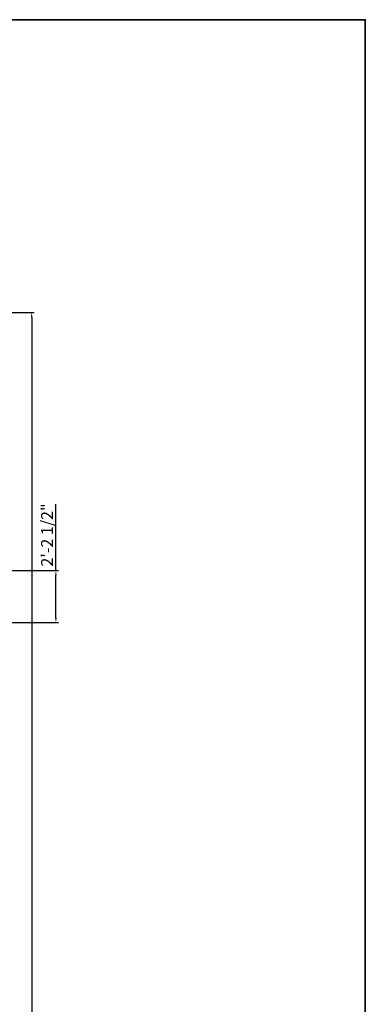
# Model space of a CAD drawing. Units: inches. Extents: x 2123 to 2977, y 1464 to 2698.
# Tile 10 of 10: x 2801 to 2977, y 2196 to 2698. Entities that reach past the tile are written whole.
import ezdxf

# ---------------------------------------------------------------- set-up
doc = ezdxf.new("R2010")
doc.units = ezdxf.units.IN
doc.layers.add('A-ANNO-DIMS', color=2, linetype='Continuous', lineweight=18)
doc.layers.add('A-ANNO-TTLB', color=7, linetype='Continuous', lineweight=35)
doc.styles.get("Standard").update_dxf_attribs({"font": 'arial.ttf'})
doc.dimstyles.new('ISO-25', dxfattribs={"dimtxt": 6, "dimasz": 2.5, "dimexe": 1.25, "dimexo": 0.625, "dimtad": 1, "dimdec": 0, "dimlunit": 3, "dimtxsty": 'Standard', "dimcen": 2.5, "dimadec": 0, "dimazin": 0, "dimtfac": 1, "dimtdec": 0, "dimtmove": 0, "dimatfit": 3, "dimfxl": 1, "dimarcsym": 0})

# ---------------------------------------------------------------- blocks, each defined once
blk = doc.blocks.new('*D9')
at = {"layer": 'A-ANNO-DIMS', "color": 0, "lineweight": -2, "transparency": 16777216}
for p, q in [((2767.56, 2548.37), (2808.58, 2548.37)), ((2807.33, 2545.87), (2807.33, 1686.46)), ((2767.56, 1683.96), (2808.58, 1683.96))]:
    blk.add_line(p, q, dxfattribs=at)
at = {"layer": 'A-ANNO-DIMS', "color": 0, "transparency": 16777216}
for points in [[(2806.91, 2545.87), (2807.74, 2545.87), (2807.33, 2548.37)], [(2806.91, 1686.46), (2807.74, 1686.46), (2807.33, 1683.96)]]:
    blk.add_solid(points, dxfattribs=at)
at = {"layer": 'Defpoints', "color": 0, "transparency": 16777216}
for p in [(2766.94, 2548.37), (2766.94, 1683.96), (2807.33, 1683.96)]:
    blk.add_point(p, dxfattribs=at)
at = {"layer": 'A-ANNO-DIMS', "color": 0, "transparency": 16777216, "insert": (2803.69, 2116.16), "char_height": 6, "attachment_point": 5, "rotation": 90}
blk.add_mtext("72'", dxfattribs=at)
blk = doc.blocks.new('*D59')
at = {"layer": 'A-ANNO-DIMS', "color": 0, "lineweight": -2, "transparency": 16777216}
for p, q in [((2819.64, 2416.87), (2819.64, 2450.65)), ((2376.14, 2416.87), (2820.89, 2416.87)), ((2819.64, 2392.84), (2819.64, 2414.37)), ((2344.56, 2390.34), (2820.89, 2390.34))]:
    blk.add_line(p, q, dxfattribs=at)
at = {"layer": 'A-ANNO-DIMS', "color": 0, "transparency": 16777216}
for points in [[(2819.22, 2414.37), (2820.05, 2414.37), (2819.64, 2416.87)], [(2819.22, 2392.84), (2820.05, 2392.84), (2819.64, 2390.34)]]:
    blk.add_solid(points, dxfattribs=at)
at = {"layer": 'Defpoints', "color": 0, "transparency": 16777216}
for p in [(2375.52, 2416.87), (2819.64, 2416.87), (2343.94, 2390.34)]:
    blk.add_point(p, dxfattribs=at)
at = {"layer": 'A-ANNO-DIMS', "color": 0, "transparency": 16777216, "insert": (2815.91, 2435.01), "char_height": 6, "attachment_point": 5, "rotation": 90}
blk.add_mtext('2\'-2 1/2"', dxfattribs=at)

msp = doc.modelspace()

# ---------------------------------------------------------------- linework, layer by layer
at = {"layer": 'A-ANNO-TTLB'}
msp.add_lwpolyline([(2123.3, 2697.62), (2977.18, 2697.62), (2977.18, 1463.53), (2123.3, 1463.53)], close=True, dxfattribs=at)

# ---------------------------------------------------------------- dimensions: what is measured, and where the dimension line sits
at = {"layer": 'A-ANNO-DIMS'}
for base, p1, p2, override, picture, middle in [((2807.33, 1683.96), (2766.94, 2548.37), (2766.94, 1683.96), {"dimclrd": 0, "dimclre": 0, "dimclrt": 0}, '*D9', (2803.69, 2116.16)), ((2819.64, 2416.87), (2343.94, 2390.34), (2375.52, 2416.87), {"dimdec": 1, "dimlfac": 1, "dimrnd": 0, "dimzin": 1, "dimdsep": 46, "dimlunit": 4, "dimfrac": 2}, '*D59', (2815.91, 2435.01))]:
    dim = msp.add_linear_dim(base=base, p1=p1, p2=p2, angle=90, dimstyle='ISO-25', override=override, dxfattribs=at)
    dim.commit()
    dim.dimension.update_dxf_attribs({"geometry": picture, "text_midpoint": middle})

doc.saveas('drawing.dxf')
